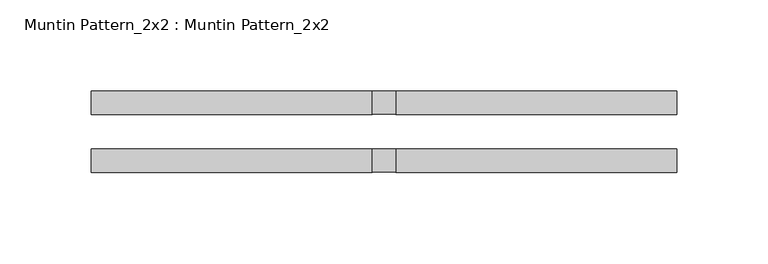
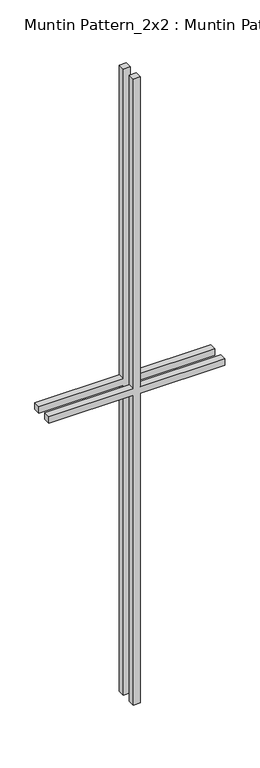
"""IFC4 building model written with IfcOpenShell, lengths in millimetres: proxy geometry, Muntin Pattern_2x2 : Muntin Pattern_2x2."""

from ifc_helpers import new_model, si_unit, frame, origin, place, context, project, spatial, polyline, outline, extrude, source, transform, mapped, element, save


def muntin_pattern_2x2_muntin_pattern_2x2_9b64c8d5(model_context):
    return source(origin(), model_context, "Body", "SweptSolid", [
        extrude(outline(polyline([(609.6, -6.35), (609.6, -160.3375), (596.9, -160.3375), (596.9, -6.35), (0.0, -6.35), (0.0, 6.35), (596.9, 6.35), (596.9, 160.3375), (609.6, 160.3375), (609.6, 6.35), (1206.5, 6.35), (1206.5, -6.35), (609.6, -6.35)])), frame((0.0, 9.525, 0.0), z_axis=(0.0, 1.0, 0.0), x_axis=(0.0, 0.0, 1.0)), (0.0, 0.0, 1.0), 12.7),
        extrude(outline(polyline([(609.6, -6.35), (609.6, -160.3375), (596.9, -160.3375), (596.9, -6.35), (0.0, -6.35), (0.0, 6.35), (596.9, 6.35), (596.9, 160.3375), (609.6, 160.3375), (609.6, 6.35), (1206.5, 6.35), (1206.5, -6.35), (609.6, -6.35)])), frame((0.0, -22.225, 0.0), z_axis=(0.0, 1.0, 0.0), x_axis=(0.0, 0.0, 1.0)), (0.0, 0.0, 1.0), 12.7),
    ])


if __name__ == "__main__":
    model = new_model("IFC4")
    model_context = context("Model", 3, world=origin())
    ifc_project = project(units=[si_unit("LENGTHUNIT", "METRE", prefix="MILLI")], contexts=[model_context])
    site = spatial("IfcSite", under=ifc_project)
    building = spatial("IfcBuilding", under=site)
    placement = place(None, origin())
    muntin_pattern_2x2_muntin_pattern_2x2_shape = muntin_pattern_2x2_muntin_pattern_2x2_9b64c8d5(model_context)
    element("IfcBuildingElementProxy", 1, Name="Muntin Pattern_2x2 : Muntin Pattern_2x2", ObjectType="Muntin Pattern_2x2 : Muntin Pattern_2x2", at=placement, inside=building, context=model_context, shape_type="MappedRepresentation", body=[
        mapped(muntin_pattern_2x2_muntin_pattern_2x2_shape, transform((0.0, 0.0, 0.0), x_axis=(1.0, 0.0, 0.0), y_axis=(0.0, 1.0, 0.0), z_axis=(0.0, 0.0, 1.0))),
    ])
    save(model, "model.ifc")

# Revit data of these elements
# Type "Muntin Pattern_2x2 : Muntin Pattern_2x2"
#   Width [instance default] = 4' - 0"
#   Thickness = 0' - 0 1/2"
#   Height [instance default] = 4' - 0"
#   Distance = 0' - 0 3/4"
#   Interior Material [instance default] = none
#   Exterior Material [instance default] = none
#   Default Elevation = 0
# Element 1 (IfcBuildingElementProxy, "Muntin Pattern_2x2 : Muntin Pattern_2x2")
#   Width = 1' - 0 5/8"
#   Height = 3' - 11 1/2"
#   Interior Material = Wood - Stained
#   Exterior Material = Clad - White
#   Materials on its faces: "Clad - White", "Wood - Stained"
# Materials
#   "Clad - White": class "Wood", colour RGB 242 242 238, transparency 0, Cost = 0
#   "Wood - Stained": class "Wood", colour RGB 224 178 126, transparency 0, Cost = 0
